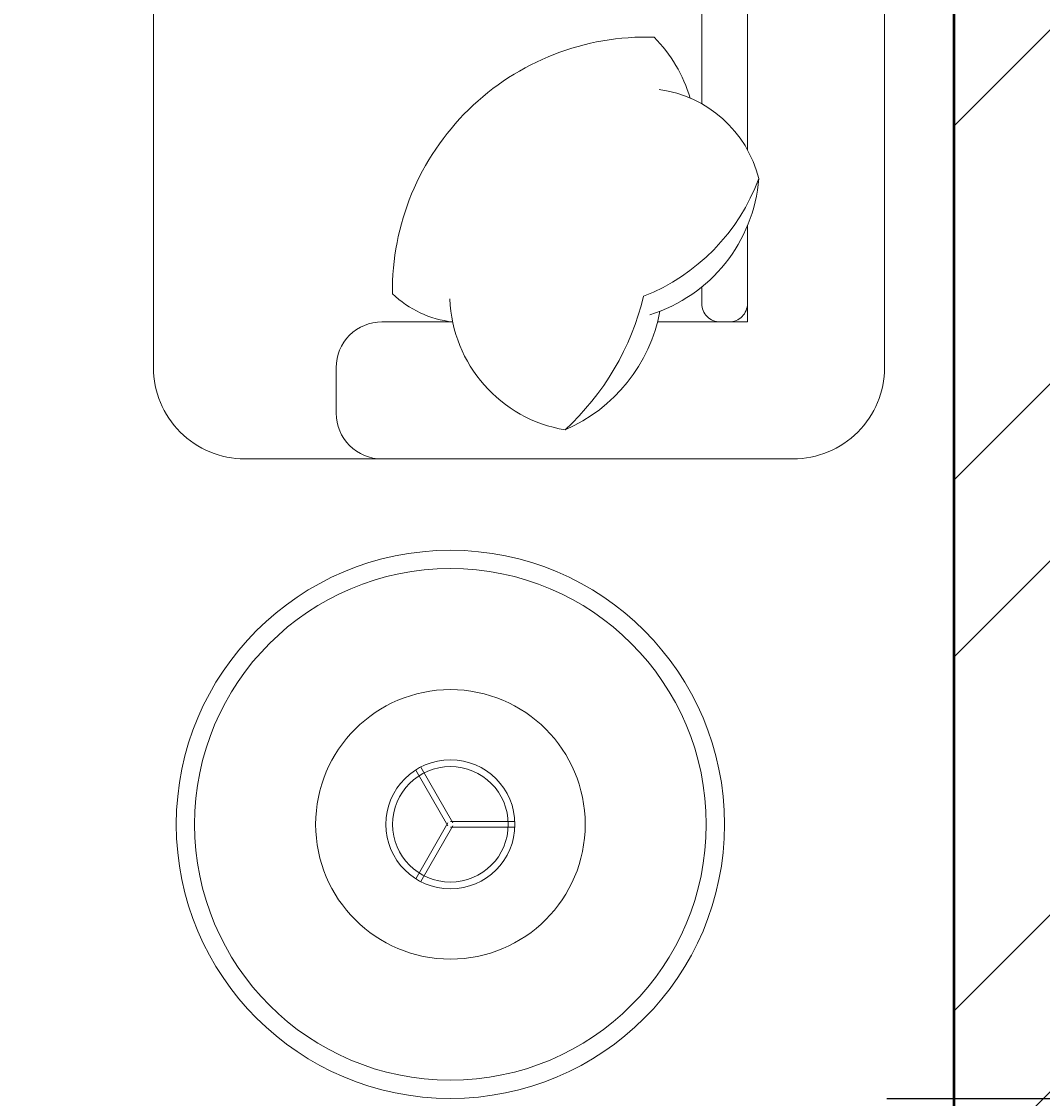
# Model space of a CAD drawing. Units: inches. Extents: x 963 to 2075, y 289 to 2657.
# Tile 21 of 98: x 1485 to 1511, y 1735 to 1763. Entities that reach past the tile are written whole.
import ezdxf

# ---------------------------------------------------------------- set-up
doc = ezdxf.new("R2010")
doc.units = ezdxf.units.IN
for name, color, linetype, lineweight in [('A-ANNO-DIMS', 2, 'Continuous', 18), ('A-FURN', 8, 'Continuous', 18), ('A-WALL', 7, 'Continuous', 50), ('A-WALL-PATT', 8, 'Continuous', 13)]:
    doc.layers.add(name, color=color, linetype=linetype, lineweight=lineweight)
doc.styles.get("Standard").update_dxf_attribs({"font": 'arial.ttf'})
doc.dimstyles.get("Standard").update_dxf_attribs({"dimtxt": 0.18, "dimasz": 0.18, "dimexe": 0.18, "dimexo": 0.0625, "dimgap": 0.09, "dimtad": 0, "dimtih": 1, "dimtoh": 1, "dimdec": 4, "dimzin": 0, "dimdsep": 46, "dimtxsty": 'Standard', "dimcen": 0.09, "dimadec": 0, "dimazin": 0, "dimtfac": 1, "dimtdec": 4, "dimtofl": 0, "dimtmove": 0, "dimatfit": 3, "dimfxl": 1, "dimtolj": 1, "dimtzin": 0, "dimarcsym": 0})

# ---------------------------------------------------------------- blocks, each defined once
blk = doc.blocks.new('SOFA-3SEAT')
at = {"ltscale": 0.03}
for p, q in [((7.593, 7.119), (6.776, 8.534)), ((7.719, 7.192), (6.902, 8.607)), ((7.593, 7.192), (6.776, 5.776)), ((7.719, 7.119), (6.902, 5.703)), ((7.656, 7.228), (9.29, 7.228)), ((7.656, 7.082), (9.29, 7.082))]:
    blk.add_line(p, q, dxfattribs=at)
blk.add_lwpolyline([(2.442, 16.426, -0.414214), (0.124, 18.743), (0.124, 32.649, -0.414214), (1.283, 33.808, -0.414214), (0.124, 34.967), (0.124, 46.555, -0.414214), (1.283, 47.713, -0.414214), (0.124, 48.872), (0.124, 62.778, -0.414214), (2.442, 65.095), (16.347, 65.095, -0.414214), (18.665, 62.778), (18.665, 18.743, -0.414214), (16.347, 16.426)], format="xyb", close=True, dxfattribs=at)
for points in [[(15.189, 24.268), (15.189, 51.011)], [(12.911, 19.902), (15.189, 19.902), (15.189, 22.34)]]:
    blk.add_lwpolyline(points)
for points in [[(15.189, 24.268), (15.189, 33.344, 0.414214), (14.725, 33.808), (14.493, 33.808, 0.414214), (14.03, 33.344), (14.03, 25.435, 0.414214)], [(7.714, 19.9, -0.165541), (6.183, 20.616, -0.425989), (12.821, 27.124, -0.121523), (13.736, 25.58, 7.115464)], [(12.714, 20.082, 0.306663), (15.477, 23.538, 0.30633), (12.954, 25.796, -0.872847)], [(10.564, 17.163, 0.14773), (12.556, 20.55, 0.213343), (15.477, 23.538, 0.178662)], [(15.189, 20.366), (15.189, 22.34, 0.414214)], [(14.03, 20.786), (14.03, 20.366, 0.414214), (14.493, 19.902), (14.725, 19.902, 0.414214), (15.189, 20.366)], [(7.643, 20.484, 0.356772), (10.564, 17.163, 0.249542), (12.971, 20.172, -9.61688)], [(5.918, 16.426, -0.414214), (4.759, 17.584), (4.759, 18.743, -0.414214), (5.918, 19.902), (7.713, 19.902)]]:
    blk.add_lwpolyline(points, format="xyb")
for radius in [6.953, 3.418, 1.636, 1.466]:
    blk.add_circle((7.656, 7.155), radius, dxfattribs=at)
blk.add_circle((7.656, 7.155), 6.489)
blk = doc.blocks.new('*D28')
at = {"layer": 'A-ANNO-DIMS', "color": 0, "lineweight": -2, "transparency": 16777216}
for p, q in [((1506.727, 1816.319), (1519.012, 1816.319)), ((1518.832, 1816.139), (1518.832, 1775.944)), ((1518.832, 1735.382), (1518.832, 1775.577)), ((1506.727, 1735.202), (1519.012, 1735.202))]:
    blk.add_line(p, q, dxfattribs=at)
at = {"layer": 'A-ANNO-DIMS', "color": 0, "transparency": 16777216}
for points in [[(1518.802, 1816.139), (1518.862, 1816.139), (1518.832, 1816.319)], [(1518.802, 1735.382), (1518.862, 1735.382), (1518.832, 1735.202)]]:
    blk.add_solid(points, dxfattribs=at)
at = {"layer": 'Defpoints', "color": 0, "transparency": 16777216}
for p in [(1506.665, 1816.319), (1518.832, 1816.319), (1506.665, 1735.202)]:
    blk.add_point(p, dxfattribs=at)
at = {"layer": 'A-ANNO-DIMS', "color": 0, "transparency": 16777216, "insert": (1518.832, 1775.761), "char_height": 0.18, "attachment_point": 5}
blk.add_mtext('\\A1;3-SEAT SOFA 81 TYP.', dxfattribs=at)

msp = doc.modelspace()

# ---------------------------------------------------------------- hatches: boundary and pattern name
at = {"layer": 'A-WALL-PATT'}
h = msp.add_hatch(dxfattribs=at)
h.set_pattern_fill('ANSI32', color=256)
h.paths.add_polyline_path([(1473.609, 2163.068), (1473.609, 2165.318), (1376.422, 2165.318), (1376.422, 2227.983), (1371.922, 2227.983), (1371.922, 2214.818), (1368.405, 2214.818), (1368.405, 2210.318), (1371.922, 2210.318), (1371.922, 2160.818), (1395.922, 2160.818), (1395.922, 2090.318), (1217.345, 2090.318), (1217.345, 2085.818), (1395.922, 2085.818), (1458.922, 2085.818), (1458.922, 2108.318), (1454.422, 2108.318), (1454.422, 2090.318), (1400.422, 2090.318), (1400.422, 2160.818), (1473.609, 2160.818)])
h.paths.add_polyline_path([(1649.422, 2210.318), (1653.225, 2210.318), (1653.225, 2214.818), (1649.422, 2214.818), (1649.422, 2227.983), (1644.922, 2227.983), (1644.922, 2165.318), (1550.099, 2165.318), (1550.099, 2160.818), (1620.922, 2160.818), (1620.922, 2112.818), (1555.446, 2112.818), (1555.446, 2108.318), (1584.327, 2108.318), (1584.327, 2084.916), (1588.827, 2084.916), (1588.827, 2108.318), (1625.422, 2108.318), (1667.951, 2108.318), (1667.951, 2022.667), (1588.827, 2022.667), (1588.827, 2047.408), (1584.327, 2047.408), (1584.327, 1996.003), (1588.827, 1996.003), (1588.827, 2018.318), (1667.951, 2018.167), (1667.951, 1928.318), (1625.422, 1928.318), (1625.422, 1923.818), (1672.451, 1923.818), (1672.451, 1928.318), (1672.451, 1946.663), (1785.446, 1946.663), (1785.446, 1951.163), (1743.034, 1951.163), (1743.034, 2017.922), (1841.422, 2017.922), (1841.422, 2014.775), (1845.922, 2014.775), (1845.922, 2017.922), (1905.922, 2017.922), (1905.922, 1987.511), (1910.422, 1987.511), (1910.422, 2022.422), (1910.422, 2068.517), (1905.922, 2068.517), (1905.922, 2022.422), (1845.922, 2022.422), (1845.922, 2025.851), (1843.672, 2025.851), (1841.422, 2025.851), (1841.422, 2022.422), (1743.034, 2022.422), (1743.034, 2084.031), (1768.451, 2084.031), (1785.446, 2084.031), (1785.446, 2088.531), (1672.451, 2088.531), (1672.451, 2112.818), (1667.951, 2112.818), (1625.422, 2112.818), (1625.422, 2160.818), (1649.422, 2160.818)])
h.paths.add_polyline_path([(1672.451, 2084.031), (1738.534, 2084.031), (1738.534, 1951.163), (1672.451, 1951.163)], flags=16)
h.paths.add_polyline_path([(1672.451, 2084.031), (1738.534, 2084.031), (1705.492, 2017.597)], flags=0)
h.paths.add_polyline_path([(1262.766, 2085.818), (1258.266, 2085.818), (1258.266, 2023.278), (1184.422, 2023.278), (1184.422, 2018.778), (1258.266, 2018.778), (1258.266, 1950.818), (1262.766, 1950.818)])
h.paths.add_polyline_path([(1312.266, 2085.818), (1307.766, 2085.818), (1307.766, 1950.818), (1312.266, 1950.818)])
h.paths.add_polyline_path([(1458.922, 1950.818), (1395.922, 1950.818), (1216.568, 1950.818), (1216.568, 1946.318), (1346.422, 1946.318), (1395.922, 1946.318), (1395.922, 1875.818), (1371.922, 1875.818), (1371.922, 1826.318), (1368.931, 1826.318), (1368.931, 1821.818), (1371.922, 1821.818), (1371.922, 1813.622), (1376.422, 1813.622), (1376.422, 1871.318), (1474.504, 1871.318), (1474.504, 1873.568), (1474.504, 1875.818), (1400.422, 1875.818), (1400.422, 1946.318), (1454.422, 1946.318), (1454.422, 1928.318), (1458.922, 1928.318)])
h.paths.add_polyline_path([(1184.422, 2120.778), (1167.922, 2120.778), (1167.922, 2134.812), (1165.672, 2134.812), (1163.422, 2134.812), (1163.422, 2120.778), (1119.922, 2120.778), (1119.922, 2098.095), (1124.422, 2098.095), (1124.422, 2116.278), (1167.922, 2116.278), (1179.922, 2116.278), (1179.922, 2045.916), (1184.422, 2045.916), (1184.422, 2090.318), (1184.422, 2116.278)])
h.paths.add_polyline_path([(1124.422, 2018.778), (1179.922, 2018.778), (1179.922, 2016.294), (1184.422, 2016.294), (1184.422, 2023.278), (1184.422, 2026.588), (1182.172, 2026.588), (1179.922, 2026.588), (1179.922, 2023.278), (1124.422, 2023.278), (1124.422, 2074.095), (1119.922, 2074.095), (1119.922, 2018.778), (1119.922, 1979.633), (1124.422, 1979.633)])
h.paths.add_polyline_path([(1184.422, 1925.778), (1184.422, 1946.318), (1184.422, 1996.073), (1182.172, 1996.073), (1179.922, 1996.073), (1179.922, 1925.778), (1124.422, 1925.778), (1124.422, 1955.633), (1119.922, 1955.502), (1119.922, 1921.278), (1158.922, 1921.278), (1158.922, 1909.983), (1163.422, 1909.983), (1163.422, 1921.278), (1184.422, 1921.278)])
h.paths.add_polyline_path([(1341.449, 1826.318), (1163.422, 1826.318), (1163.422, 1849.983), (1158.922, 1849.983), (1158.922, 1821.818), (1158.922, 1804.033), (1163.422, 1804.033), (1163.422, 1821.818), (1341.449, 1821.818)])
h.paths.add_polyline_path([(1222.981, 1713.818), (1163.422, 1713.818), (1163.422, 1744.033), (1161.172, 1744.033), (1158.922, 1744.033), (1158.922, 1713.818), (1119.922, 1713.818), (1119.922, 1694.65), (1124.422, 1694.65), (1124.422, 1709.318), (1158.922, 1709.318), (1222.981, 1709.318)])
h.paths.add_polyline_path([(1328.422, 1713.818), (1252.042, 1713.818), (1252.042, 1711.568), (1252.042, 1709.318), (1256.422, 1709.318), (1256.422, 1547.318), (1232.937, 1547.318), (1232.937, 1545.068), (1232.937, 1542.818), (1292.422, 1542.818), (1292.422, 1527.634), (1296.922, 1527.634), (1296.922, 1542.818), (1299.464, 1542.818), (1299.464, 1547.318), (1260.922, 1547.318), (1260.922, 1658.318), (1343.661, 1658.318), (1343.661, 1660.568), (1343.661, 1662.818), (1328.422, 1662.818), (1328.422, 1676.589), (1327.402, 1676.589), (1323.922, 1676.589), (1323.922, 1662.818), (1260.922, 1662.818), (1260.922, 1709.318), (1323.922, 1709.318), (1323.922, 1699.851), (1328.422, 1699.851)])
h.paths.add_polyline_path([(1649.422, 1875.818), (1625.422, 1875.818), (1625.422, 1928.318), (1620.922, 1928.318), (1588.827, 1928.318), (1588.827, 1950.59), (1584.327, 1950.59), (1584.327, 1928.318), (1555.446, 1928.318), (1555.446, 1923.818), (1620.922, 1923.818), (1620.922, 1875.818), (1548.952, 1875.818), (1548.952, 1873.568), (1548.952, 1871.318), (1644.922, 1871.318), (1644.922, 1813.622), (1649.422, 1813.622), (1649.422, 1821.818), (1652.045, 1821.818), (1652.045, 1824.068), (1652.045, 1826.318), (1649.422, 1826.318)])
h.paths.add_polyline_path([(1512.922, 1871.318), (1516.476, 1871.318), (1516.476, 1875.818), (1512.922, 1875.818), (1512.922, 1923.818), (1512.922, 1928.318), (1512.922, 1930.827), (1508.422, 1930.827), (1508.422, 1875.818), (1504.411, 1875.818), (1504.411, 1871.318), (1508.422, 1871.318), (1508.422, 1713.818), (1376.422, 1713.818), (1376.422, 1743.325), (1371.922, 1743.325), (1371.922, 1709.318), (1371.922, 1706.01), (1376.422, 1706.01), (1376.422, 1709.318), (1508.422, 1709.318), (1508.422, 1547.318), (1501.871, 1547.318), (1501.871, 1542.818), (1508.422, 1542.818), (1508.422, 1482.818), (1508.422, 1436.318), (1512.922, 1436.318), (1512.922, 1542.818), (1519.318, 1542.818), (1519.318, 1545.068), (1519.318, 1547.318), (1512.922, 1547.318), (1512.922, 1709.318), (1644.922, 1709.318), (1644.922, 1707.548), (1649.422, 1707.548), (1649.422, 1709.318), (1649.422, 1743.325), (1644.922, 1743.325), (1644.922, 1713.818), (1512.922, 1713.818)])
h.paths.add_polyline_path([(1129.884, 1545.068), (1129.884, 1547.318), (1124.422, 1547.318), (1095.922, 1547.318), (1095.922, 1614.818), (1124.422, 1614.818), (1124.422, 1619.318), (1095.922, 1619.318), (1091.422, 1619.318), (1091.422, 1542.818), (1095.922, 1542.818), (1119.922, 1542.818), (1129.884, 1542.818)])
h.paths.add_polyline_path([(1208.422, 1542.818), (1211.74, 1542.818), (1211.74, 1547.318), (1198.851, 1547.318), (1198.851, 1542.818), (1203.922, 1542.818), (1203.922, 1478.318), (1208.422, 1478.318), (1296.922, 1478.318), (1296.922, 1503.634), (1292.422, 1503.634), (1292.422, 1482.818), (1208.422, 1482.818)])
h.paths.add_polyline_path([(1430.422, 1542.818), (1435.699, 1542.818), (1435.699, 1545.068), (1435.699, 1547.318), (1422.658, 1547.318), (1422.658, 1545.068), (1422.658, 1542.818), (1425.922, 1542.818), (1425.922, 1482.857), (1341.922, 1482.857), (1341.922, 1502.732), (1337.422, 1502.732), (1337.422, 1478.357), (1425.922, 1478.357), (1425.922, 1440.818), (1425.922, 1436.318), (1430.422, 1436.318)])
h.paths.add_polyline_path([(1698.482, 2004.259), (1727.695, 2004.259), (1727.695, 2022.916), (1698.482, 2022.916)], flags=8)

# ---------------------------------------------------------------- linework, layer by layer
at = {"layer": 'A-WALL'}
msp.add_line((1508.422, 1871.318), (1508.422, 1713.818), dxfattribs=at)

# ---------------------------------------------------------------- block references
at = {"layer": 'A-FURN'}
msp.add_blockref('SOFA-3SEAT', (1488, 1735), dxfattribs=at)

# ---------------------------------------------------------------- dimensions: what is measured, and where the dimension line sits
at = {"layer": 'A-ANNO-DIMS'}
dim = msp.add_linear_dim(base=(1518.832, 1816.319), p1=(1506.665, 1735.202), p2=(1506.665, 1816.319), angle=90, text='3-SEAT SOFA <> TYP.', dimstyle='Standard', override={"dimdec": 0, "dimlfac": 1, "dimrnd": 0, "dimzin": 0, "dimdsep": 46, "dimlunit": 2}, dxfattribs=at)
dim.commit()
dim.dimension.update_dxf_attribs({"geometry": '*D28', "text_midpoint": (1518.832, 1775.761)})

doc.saveas('drawing.dxf')
